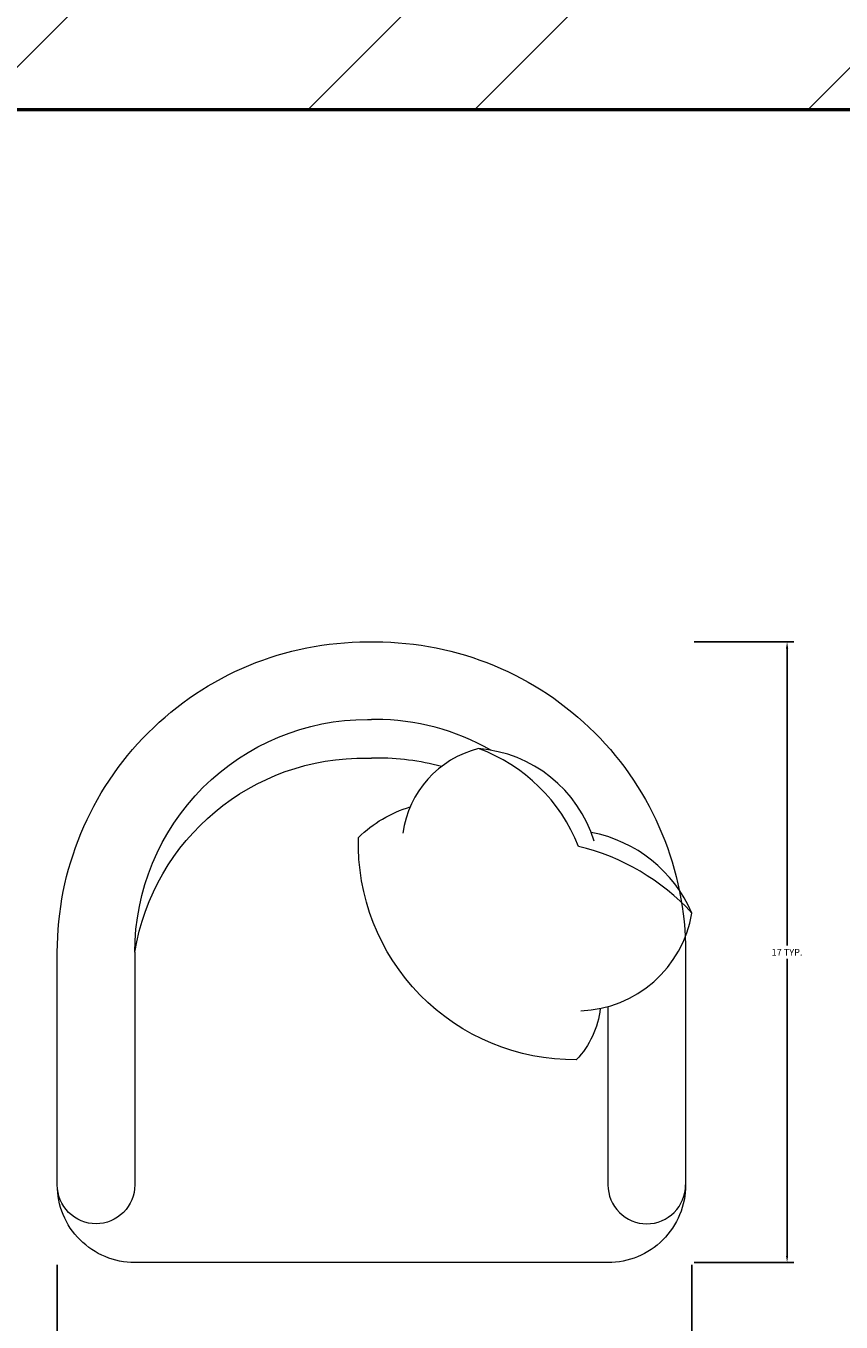
# Model space of a CAD drawing. Units: inches. Extents: x 963 to 2075, y 289 to 2657.
# Tile 78 of 98: x 1467 to 1489, y 2290 to 2325. Entities that reach past the tile are written whole.
import ezdxf

# ---------------------------------------------------------------- set-up
doc = ezdxf.new("R2010")
doc.units = ezdxf.units.IN
for name, color, linetype, lineweight in [('A-ANNO-DIMS', 2, 'Continuous', 18), ('A-FURN', 8, 'Continuous', 18), ('A-WALL', 7, 'Continuous', 50), ('A-WALL-PATT', 8, 'Continuous', 13)]:
    doc.layers.add(name, color=color, linetype=linetype, lineweight=lineweight)
doc.styles.get("Standard").update_dxf_attribs({"font": 'arial.ttf'})
doc.dimstyles.get("Standard").update_dxf_attribs({"dimtxt": 0.18, "dimasz": 0.18, "dimexe": 0.18, "dimexo": 0.0625, "dimgap": 0.09, "dimtad": 0, "dimtih": 1, "dimtoh": 1, "dimdec": 4, "dimzin": 0, "dimdsep": 46, "dimtxsty": 'Standard', "dimcen": 0.09, "dimadec": 0, "dimazin": 0, "dimtfac": 1, "dimtdec": 4, "dimtofl": 0, "dimtmove": 0, "dimatfit": 3, "dimfxl": 1, "dimtolj": 1, "dimtzin": 0, "dimarcsym": 0})

# ---------------------------------------------------------------- blocks, each defined once
blk = doc.blocks.new('ARMCHAIR-B')
at = {"ltscale": 0.03}
blk.add_lwpolyline([(8.888, -0.236), (2.514, -0.236, -0.414214), (0.425, 1.854), (0.425, 8.122, -0.414214), (8.783, 16.481), (8.888, 16.481), (8.992, 16.481, -0.414214), (17.351, 8.122), (17.351, 1.854, -0.414214), (15.261, -0.236), (8.888, -0.236)], format="xyb", dxfattribs=at)
for points in [[(2.514, 8.122, -0.414214), (8.783, 14.391), (8.888, 14.391)], [(12.104, 13.565, 0.130591), (8.992, 14.391), (8.888, 14.391)], [(2.514, 8.122, -0.372719), (8.783, 13.347), (8.888, 13.347)], [(10.774, 13.121, 0.072384), (8.992, 13.347), (8.888, 13.347)], [(14.89, 11.116, 0.306663), (11.774, 13.606, 0.30633), (9.738, 11.332, -0.872847)], [(17.522, 9.177, 0.14773), (14.468, 10.973, 0.213343), (11.774, 13.606, 0.178662)], [(15.054, 6.607, -0.165541), (14.408, 5.227, -0.425989), (8.54, 11.212, -0.121523), (9.933, 12.037, 7.115464)], [(14.528, 6.544, 0.356772), (17.522, 9.177, 0.249542), (14.809, 11.347, -9.61688)], [(2.514, 8.123), (2.514, 1.854, -0.414214), (1.469, 0.809), (1.469, 0.809, -0.414214), (0.425, 1.854)], [(15.261, 6.658), (15.261, 1.854, 0.414214), (16.306, 0.809), (16.306, 0.809, 0.414214), (17.351, 1.854)]]:
    blk.add_lwpolyline(points, format="xyb")
blk = doc.blocks.new('*D24')
at = {"layer": 'A-ANNO-DIMS', "color": 0, "lineweight": -2, "transparency": 16777216}
for p, q in [((1467.425, 2291.701), (1467.425, 2289.019)), ((1484.522, 2291.701), (1484.522, 2289.019)), ((1467.605, 2289.199), (1474.616, 2289.199)), ((1484.342, 2289.199), (1477.331, 2289.199))]:
    blk.add_line(p, q, dxfattribs=at)
at = {"layer": 'A-ANNO-DIMS', "color": 0, "transparency": 16777216}
for points in [[(1467.605, 2289.229), (1467.605, 2289.169), (1467.425, 2289.199)], [(1484.342, 2289.229), (1484.342, 2289.169), (1484.522, 2289.199)]]:
    blk.add_solid(points, dxfattribs=at)
at = {"layer": 'Defpoints', "color": 0, "transparency": 16777216}
for p in [(1467.425, 2291.764), (1484.522, 2291.764), (1484.522, 2289.199)]:
    blk.add_point(p, dxfattribs=at)
at = {"layer": 'A-ANNO-DIMS', "color": 0, "transparency": 16777216, "insert": (1475.973, 2289.199), "char_height": 0.18, "attachment_point": 5}
blk.add_mtext('\\A1;ARMCHAIR B 17 TYP.', dxfattribs=at)
blk = doc.blocks.new('*D25')
at = {"layer": 'A-ANNO-DIMS', "color": 0, "lineweight": -2, "transparency": 16777216}
for p, q in [((1484.584, 2308.481), (1487.266, 2308.481)), ((1487.086, 2308.301), (1487.086, 2300.303)), ((1487.086, 2291.944), (1487.086, 2299.942)), ((1484.584, 2291.764), (1487.266, 2291.764))]:
    blk.add_line(p, q, dxfattribs=at)
at = {"layer": 'A-ANNO-DIMS', "color": 0, "transparency": 16777216}
for points in [[(1487.056, 2308.301), (1487.116, 2308.301), (1487.086, 2308.481)], [(1487.056, 2291.944), (1487.116, 2291.944), (1487.086, 2291.764)]]:
    blk.add_solid(points, dxfattribs=at)
at = {"layer": 'Defpoints', "color": 0, "transparency": 16777216}
for p in [(1484.522, 2308.481), (1487.086, 2308.481), (1484.522, 2291.764)]:
    blk.add_point(p, dxfattribs=at)
at = {"layer": 'A-ANNO-DIMS', "color": 0, "transparency": 16777216, "insert": (1487.086, 2300.122), "char_height": 0.18, "attachment_point": 5}
blk.add_mtext('\\A1;17 TYP.', dxfattribs=at)

msp = doc.modelspace()

# ---------------------------------------------------------------- hatches: boundary and pattern name
at = {"layer": 'A-WALL-PATT'}
h = msp.add_hatch(dxfattribs=at)
h.set_pattern_fill('ANSI32', color=256)
h.paths.add_polyline_path([(1296.922, 2558.318), (1203.922, 2558.318), (1203.922, 2493.818), (1191.533, 2493.818), (1191.533, 2489.318), (1211.063, 2489.318), (1211.063, 2492.02), (1211.063, 2493.818), (1208.422, 2493.818), (1208.422, 2553.818), (1292.422, 2553.818), (1292.422, 2538.863), (1296.922, 2538.863)])
h.paths.add_polyline_path([(1442.422, 2558.318), (1349.422, 2558.318), (1349.422, 2538.943), (1353.922, 2538.943), (1353.922, 2553.818), (1437.922, 2553.818), (1437.922, 2493.818), (1434.542, 2493.818), (1434.542, 2489.318), (1448.311, 2489.318), (1448.311, 2491.568), (1448.311, 2493.818), (1442.422, 2493.818)])
h.paths.add_polyline_path([(1415.554, 2491.568), (1415.554, 2493.818), (1340.941, 2493.818), (1340.941, 2489.318), (1371.922, 2489.318), (1371.922, 2378.318), (1367.596, 2378.318), (1367.596, 2373.818), (1371.922, 2373.818), (1371.922, 2355.185), (1376.422, 2355.185), (1376.422, 2489.318), (1415.554, 2489.318)])
h.paths.add_polyline_path([(1304.941, 2491.568), (1304.941, 2493.818), (1296.922, 2493.818), (1296.922, 2514.863), (1292.422, 2514.863), (1292.422, 2493.818), (1232.808, 2493.818), (1232.808, 2489.318), (1256.422, 2489.318), (1256.422, 2327.318), (1253.714, 2327.318), (1253.714, 2322.818), (1328.422, 2322.818), (1328.422, 2331.147), (1323.922, 2331.147), (1323.922, 2327.318), (1260.922, 2327.318), (1260.922, 2373.818), (1323.922, 2373.818), (1323.922, 2357.812), (1328.422, 2357.812), (1328.422, 2373.818), (1346.007, 2373.818), (1346.007, 2376.068), (1346.007, 2378.318), (1260.922, 2378.318), (1260.922, 2489.318), (1304.941, 2489.318)])
h.paths.add_polyline_path([(1226.654, 2327.318), (1124.422, 2327.318), (1124.422, 2347.447), (1119.922, 2347.447), (1119.922, 2322.818), (1163.422, 2322.818), (1163.422, 2305.435), (1165.672, 2305.435), (1167.922, 2305.435), (1167.922, 2322.818), (1226.654, 2322.818), (1226.654, 2325.068)])
h.paths.add_polyline_path([(1095.922, 2489.318), (1124.422, 2489.318), (1131.533, 2489.318), (1131.533, 2491.568), (1131.533, 2493.818), (1119.922, 2493.818), (1091.422, 2493.818), (1091.422, 2417.318), (1095.922, 2417.318), (1119.922, 2417.318), (1119.922, 2407.447), (1124.422, 2407.447), (1124.422, 2421.818), (1095.922, 2421.818)])
h.paths.add_polyline_path([(1512.922, 2558.318), (1508.422, 2558.318), (1508.422, 2493.818), (1503.401, 2493.818), (1503.401, 2489.318), (1508.422, 2489.318), (1508.422, 2327.318), (1376.422, 2327.318), (1376.422, 2330.273), (1371.922, 2330.273), (1371.922, 2298.744), (1376.422, 2298.744), (1376.422, 2322.818), (1508.422, 2322.818), (1508.422, 2165.318), (1504.255, 2165.318), (1504.255, 2160.818), (1508.422, 2160.818), (1508.422, 2108.318), (1512.922, 2108.318), (1512.922, 2160.818), (1516.182, 2160.818), (1516.182, 2163.068), (1516.182, 2165.318), (1512.922, 2165.318), (1512.922, 2322.818), (1644.922, 2322.818), (1644.922, 2298.744), (1649.422, 2298.744), (1649.422, 2322.818), (1649.422, 2330.944), (1647.172, 2330.944), (1644.922, 2330.944), (1644.922, 2327.318), (1512.922, 2327.318), (1512.922, 2489.318), (1516.759, 2489.318), (1516.759, 2491.568), (1516.759, 2493.818), (1512.922, 2493.818)])
h.paths.add_polyline_path([(1671.922, 2558.318), (1578.922, 2558.318), (1578.922, 2493.818), (1573.526, 2493.818), (1573.526, 2489.318), (1586.537, 2489.318), (1586.537, 2491.568), (1586.537, 2493.818), (1583.422, 2493.818), (1583.422, 2553.818), (1667.422, 2553.818), (1667.422, 2541.109), (1671.922, 2541.109)])
h.paths.add_polyline_path([(1681.257, 2493.818), (1671.922, 2493.818), (1671.922, 2517.109), (1667.422, 2517.109), (1667.422, 2493.818), (1610.218, 2493.818), (1610.218, 2489.318), (1644.922, 2489.318), (1644.922, 2357.865), (1649.422, 2357.865), (1649.422, 2373.818), (1652.203, 2373.818), (1652.203, 2375.827), (1652.203, 2378.318), (1649.422, 2378.318), (1649.422, 2489.318), (1681.257, 2489.318), (1681.257, 2491.568)])
h.paths.add_polyline_path([(1821.922, 2558.318), (1728.922, 2558.318), (1728.922, 2541), (1733.422, 2541), (1733.422, 2553.818), (1817.422, 2553.818), (1817.422, 2493.818), (1813.507, 2493.818), (1813.507, 2489.318), (1830.078, 2489.318), (1830.078, 2491.568), (1830.078, 2493.818), (1821.922, 2493.818)])
h.paths.add_polyline_path([(1794.244, 2493.818), (1717.257, 2493.818), (1717.257, 2489.318), (1760.422, 2489.318), (1760.422, 2378.318), (1674.401, 2378.318), (1674.401, 2373.818), (1692.922, 2373.818), (1692.922, 2356.954), (1697.422, 2356.954), (1697.422, 2373.818), (1760.422, 2373.818), (1760.422, 2327.318), (1697.422, 2327.318), (1697.422, 2333.341), (1692.922, 2333.341), (1692.922, 2322.818), (1768.037, 2322.818), (1768.037, 2325.068), (1768.037, 2327.318), (1764.922, 2327.318), (1764.922, 2489.318), (1794.244, 2489.318)])
h.paths.add_polyline_path([(1733.422, 2517), (1728.922, 2517), (1728.922, 2493.818), (1733.422, 2493.818)], flags=17)
h.paths.add_polyline_path([(1929.922, 2493.818), (1890.078, 2493.818), (1890.078, 2489.318), (1896.922, 2489.318), (1925.422, 2489.318), (1925.422, 2421.818), (1896.922, 2421.818), (1896.922, 2408.318), (1901.422, 2408.318), (1901.422, 2417.318), (1925.422, 2417.318), (1929.922, 2417.318)])
h.paths.add_polyline_path([(1901.422, 2348.318), (1896.922, 2348.318), (1896.922, 2327.318), (1800.423, 2327.318), (1800.423, 2322.818), (1853.422, 2322.818), (1853.422, 2309.453), (1857.922, 2309.453), (1857.922, 2322.818), (1901.422, 2322.818)])
h.paths.add_polyline_path([(1857.922, 2249.453), (1853.422, 2249.453), (1853.422, 2214.818), (1686.309, 2214.818), (1686.309, 2210.318), (1853.422, 2210.318), (1853.422, 2202.134), (1857.922, 2202.134), (1857.922, 2210.318)])
h.paths.add_polyline_path([(1857.922, 2142.134), (1853.422, 2142.134), (1853.422, 2115.422), (1841.422, 2115.422), (1841.422, 2088.531), (1841.422, 2046.949), (1845.922, 2046.949), (1845.922, 2110.922), (1905.922, 2110.922), (1905.922, 2092.517), (1910.422, 2092.517), (1910.422, 2115.422), (1857.922, 2115.422)])
h.paths.add_polyline_path([(1532.436, 1482.342), (1573.456, 1482.342), (1573.456, 1501), (1532.436, 1501)], flags=9)
h.paths.add_polyline_path([(1438.658, 1486.302), (1479.678, 1486.302), (1479.678, 1504.96), (1438.658, 1504.96)], flags=9)
h.paths.add_polyline_path([(1411.215, 1365.308), (1659.139, 1365.308), (1659.139, 1402.401), (1411.215, 1402.401)], flags=9)
h.paths.add_polyline_path([(1185.671, 2296.298), (1248.16, 2296.298), (1248.16, 2314.955), (1185.671, 2314.955)], flags=9)
h.paths.add_polyline_path([(1177.31, 2187.35), (1216.15, 2187.35), (1216.15, 2206.007), (1177.31, 2206.007)], flags=9)
h.paths.add_polyline_path([(1295.101, 1602.083), (1328.26, 1602.083), (1328.26, 1620.741), (1295.101, 1620.741)], flags=9)
h.paths.add_polyline_path([(1525.126, 2005.99), (1558.39, 2005.99), (1558.39, 2024.648), (1525.126, 2024.648)], flags=9)
h.paths.add_polyline_path([(1459.606, 1977.125), (1472.195, 1977.125), (1472.195, 1987.429), (1459.606, 1987.429)], flags=9)
h.paths.add_polyline_path([(1467.815, 2053.676), (1480.018, 2053.676), (1480.018, 2063.979), (1467.815, 2063.979)], flags=9)
h.paths.add_polyline_path([(1555.184, 2119.02), (1584.563, 2119.02), (1584.563, 2137.678), (1555.184, 2137.678)], flags=25)
h.paths.add_polyline_path([(1405.389, 2115.291), (1444.478, 2115.291), (1444.478, 2133.948), (1405.389, 2133.948)], flags=25)
h.paths.add_polyline_path([(1698.482, 2004.259), (1727.695, 2004.259), (1727.695, 2022.916), (1698.482, 2022.916)], flags=9)
h.paths.add_polyline_path([(1612.158, 1972.855), (1629.016, 1972.855), (1629.016, 1983.159), (1612.158, 1983.159)], flags=9)
h.paths.add_polyline_path([(1608.289, 2060.036), (1625.147, 2060.036), (1625.147, 2070.34), (1608.289, 2070.34)], flags=9)
h.paths.add_polyline_path([(1527.954, 1684.402), (1566.795, 1684.402), (1566.795, 1703.06), (1527.954, 1703.06)], flags=9)
h.paths.add_polyline_path([(1422.792, 1683.59), (1461.633, 1683.59), (1461.633, 1702.247), (1422.792, 1702.247)], flags=9)
h.paths.add_polyline_path([(1531.262, 1732.459), (1574.015, 1732.459), (1574.015, 1751.116), (1531.262, 1751.116)], flags=9)
h.paths.add_polyline_path([(1402.872, 1732.845), (1439.799, 1732.845), (1439.799, 1751.502), (1402.872, 1751.502)], flags=9)
h.paths.add_polyline_path([(1243.122, 1923.132), (1281.962, 1923.132), (1281.962, 1941.79), (1243.122, 1941.79)], flags=9)
h.paths.add_polyline_path([(1181.752, 1792.268), (1244.241, 1792.268), (1244.241, 1810.926), (1181.752, 1810.926)], flags=9)
h.paths.add_polyline_path([(1265.822, 1670.3), (1316.071, 1670.3), (1316.071, 1688.957), (1265.822, 1688.957)], flags=9)
h.paths.add_polyline_path([(1140.263, 1676.054), (1179.104, 1676.054), (1179.104, 1694.711), (1140.263, 1694.711)], flags=9)
h.paths.add_polyline_path([(1107.49, 1490.889), (1143.374, 1490.889), (1143.374, 1509.546), (1107.49, 1509.546)], flags=9)
h.paths.add_polyline_path([(1217.584, 1483.899), (1246.741, 1483.899), (1246.741, 1502.556), (1217.584, 1502.556)], flags=9)
h.paths.add_polyline_path([(1389.21, 1486.919), (1418.367, 1486.919), (1418.367, 1505.576), (1389.21, 1505.576)], flags=9)
h.paths.add_polyline_path([(1672.208, 1602.083), (1705.366, 1602.083), (1705.366, 1620.741), (1672.208, 1620.741)], flags=9)
h.paths.add_polyline_path([(1752.082, 1522.638), (1781.24, 1522.638), (1781.24, 1541.295), (1752.082, 1541.295)], flags=9)
h.paths.add_polyline_path([(1848.275, 1491.26), (1884.158, 1491.26), (1884.158, 1509.918), (1848.275, 1509.918)], flags=9)
h.paths.add_polyline_path([(1822.47, 1685.62), (1861.31, 1685.62), (1861.31, 1704.278), (1822.47, 1704.278)], flags=9)
h.paths.add_polyline_path([(1713.195, 1672.232), (1763.444, 1672.232), (1763.444, 1690.889), (1713.195, 1690.889)], flags=9)
h.paths.add_polyline_path([(1736.619, 1790.578), (1799.109, 1790.578), (1799.109, 1809.235), (1736.619, 1809.235)], flags=9)
h.paths.add_polyline_path([(1691.491, 1916.355), (1730.332, 1916.355), (1730.332, 1935.013), (1691.491, 1935.013)], flags=9)
h.paths.add_polyline_path([(1764.872, 1973.922), (1794.306, 1973.922), (1794.306, 1992.58), (1764.872, 1992.58)], flags=9)
h.paths.add_polyline_path([(1767.854, 2034.017), (1797.288, 2034.017), (1797.288, 2052.674), (1767.854, 2052.674)], flags=9)
h.paths.add_polyline_path([(1851.593, 2060.331), (1880.751, 2060.331), (1880.751, 2078.989), (1851.593, 2078.989)], flags=25)
h.paths.add_polyline_path([(1688.491, 2086.874), (1727.332, 2086.874), (1727.332, 2105.531), (1688.491, 2105.531)], flags=9)
h.paths.add_polyline_path([(1537.743, 2293.581), (1580.495, 2293.581), (1580.495, 2312.239), (1537.743, 2312.239)], flags=25)
h.paths.add_polyline_path([(1425.587, 2296.109), (1468.34, 2296.109), (1468.34, 2314.766), (1425.587, 2314.766)], flags=25)
h.paths.add_polyline_path([(1278.518, 2004.184), (1307.72, 2004.184), (1307.72, 2022.841), (1278.518, 2022.841)], flags=9)
h.paths.add_polyline_path([(1193.282, 1973.635), (1222.715, 1973.635), (1222.715, 1992.292), (1193.282, 1992.292)], flags=9)
h.paths.add_polyline_path([(1192.411, 2040.577), (1221.845, 2040.577), (1221.845, 2059.234), (1192.411, 2059.234)], flags=9)
h.paths.add_polyline_path([(1130.603, 1951.393), (1159.76, 1951.393), (1159.76, 1970.05), (1130.603, 1970.05)], flags=9)
h.paths.add_polyline_path([(1132.827, 2052.494), (1161.984, 2052.494), (1161.984, 2071.151), (1132.827, 2071.151)], flags=9)
h.paths.add_polyline_path([(1265.128, 2334.619), (1315.377, 2334.619), (1315.377, 2353.277), (1265.128, 2353.277)], flags=25)
h.paths.add_polyline_path([(1136.741, 2330.785), (1175.582, 2330.785), (1175.582, 2349.443), (1136.741, 2349.443)], flags=9)
h.paths.add_polyline_path([(1287.422, 2417.204), (1320.58, 2417.204), (1320.58, 2435.861), (1287.422, 2435.861)], flags=25)
h.paths.add_polyline_path([(1430.988, 2329.159), (1469.828, 2329.159), (1469.828, 2347.816), (1430.988, 2347.816)], flags=25)
h.paths.add_polyline_path([(1525.424, 2329.213), (1564.264, 2329.213), (1564.264, 2347.87), (1525.424, 2347.87)], flags=25)
h.paths.add_polyline_path([(1684.525, 2382.799), (1717.683, 2382.799), (1717.683, 2401.457), (1684.525, 2401.457)], flags=25)
h.paths.add_polyline_path([(1704.805, 2340.293), (1755.054, 2340.293), (1755.054, 2358.95), (1704.805, 2358.95)], flags=25)
h.paths.add_polyline_path([(1694.113, 2287.757), (1756.602, 2287.757), (1756.602, 2306.414), (1694.113, 2306.414)], flags=9)
h.paths.add_polyline_path([(1815.778, 2329.861), (1854.618, 2329.861), (1854.618, 2348.518), (1815.778, 2348.518)], flags=9)
h.paths.add_polyline_path([(1842.873, 2514.256), (1878.756, 2514.256), (1878.756, 2532.914), (1842.873, 2532.914)], flags=9)
h.paths.add_polyline_path([(1769.513, 2531.447), (1798.671, 2531.447), (1798.671, 2550.104), (1769.513, 2550.104)], flags=25)
h.paths.add_polyline_path([(1594.772, 2518.468), (1623.93, 2518.468), (1623.93, 2537.125), (1594.772, 2537.125)], flags=25)
h.paths.add_polyline_path([(1520.723, 2516.185), (1556.606, 2516.185), (1556.606, 2534.842), (1520.723, 2534.842)], flags=25)
h.paths.add_polyline_path([(1464.456, 2516.694), (1500.34, 2516.694), (1500.34, 2535.351), (1464.456, 2535.351)], flags=25)
h.paths.add_polyline_path([(1365.696, 2528.97), (1394.854, 2528.97), (1394.854, 2547.627), (1365.696, 2547.627)], flags=25)
h.paths.add_polyline_path([(1222.838, 2516.231), (1251.995, 2516.231), (1251.995, 2534.889), (1222.838, 2534.889)], flags=25)
h.paths.add_polyline_path([(1104.545, 2509.6), (1140.429, 2509.6), (1140.429, 2528.257), (1104.545, 2528.257)], flags=9)
h = msp.add_hatch(dxfattribs=at)
h.set_pattern_fill('ANSI32', color=256)
h.paths.add_polyline_path([(1335.968, 2212.568), (1335.968, 2214.818), (1167.922, 2214.818), (1167.922, 2245.435), (1163.422, 2245.435), (1163.422, 2210.318), (1163.422, 2194.812), (1167.922, 2194.812), (1167.922, 2210.318), (1335.968, 2210.318)])
h.paths.add_polyline_path([(1532.436, 1482.342), (1573.456, 1482.342), (1573.456, 1501), (1532.436, 1501)], flags=9)
h.paths.add_polyline_path([(1438.658, 1486.302), (1479.678, 1486.302), (1479.678, 1504.96), (1438.658, 1504.96)], flags=9)
h.paths.add_polyline_path([(1411.215, 1365.308), (1659.139, 1365.308), (1659.139, 1402.401), (1411.215, 1402.401)], flags=9)
h.paths.add_polyline_path([(1185.671, 2296.298), (1248.16, 2296.298), (1248.16, 2314.955), (1185.671, 2314.955)], flags=9)
h.paths.add_polyline_path([(1177.31, 2187.35), (1216.15, 2187.35), (1216.15, 2206.007), (1177.31, 2206.007)], flags=9)
h.paths.add_polyline_path([(1295.101, 1602.083), (1328.26, 1602.083), (1328.26, 1620.741), (1295.101, 1620.741)], flags=9)
h.paths.add_polyline_path([(1525.126, 2005.99), (1558.39, 2005.99), (1558.39, 2024.648), (1525.126, 2024.648)], flags=9)
h.paths.add_polyline_path([(1459.606, 1977.125), (1472.195, 1977.125), (1472.195, 1987.429), (1459.606, 1987.429)], flags=9)
h.paths.add_polyline_path([(1467.815, 2053.676), (1480.018, 2053.676), (1480.018, 2063.979), (1467.815, 2063.979)], flags=9)
h.paths.add_polyline_path([(1555.184, 2119.02), (1584.563, 2119.02), (1584.563, 2137.678), (1555.184, 2137.678)], flags=9)
h.paths.add_polyline_path([(1405.389, 2115.291), (1444.478, 2115.291), (1444.478, 2133.948), (1405.389, 2133.948)], flags=9)
h.paths.add_polyline_path([(1698.482, 2004.259), (1727.695, 2004.259), (1727.695, 2022.916), (1698.482, 2022.916)], flags=9)
h.paths.add_polyline_path([(1612.158, 1972.855), (1629.016, 1972.855), (1629.016, 1983.159), (1612.158, 1983.159)], flags=9)
h.paths.add_polyline_path([(1608.289, 2060.036), (1625.147, 2060.036), (1625.147, 2070.34), (1608.289, 2070.34)], flags=9)
h.paths.add_polyline_path([(1527.954, 1684.402), (1566.795, 1684.402), (1566.795, 1703.06), (1527.954, 1703.06)], flags=9)
h.paths.add_polyline_path([(1422.792, 1683.59), (1461.633, 1683.59), (1461.633, 1702.247), (1422.792, 1702.247)], flags=9)
h.paths.add_polyline_path([(1531.262, 1732.459), (1574.015, 1732.459), (1574.015, 1751.116), (1531.262, 1751.116)], flags=9)
h.paths.add_polyline_path([(1402.872, 1732.845), (1439.799, 1732.845), (1439.799, 1751.502), (1402.872, 1751.502)], flags=9)
h.paths.add_polyline_path([(1243.122, 1923.132), (1281.962, 1923.132), (1281.962, 1941.79), (1243.122, 1941.79)], flags=9)
h.paths.add_polyline_path([(1181.752, 1792.268), (1244.241, 1792.268), (1244.241, 1810.926), (1181.752, 1810.926)], flags=9)
h.paths.add_polyline_path([(1265.822, 1670.3), (1316.071, 1670.3), (1316.071, 1688.957), (1265.822, 1688.957)], flags=9)
h.paths.add_polyline_path([(1140.263, 1676.054), (1179.104, 1676.054), (1179.104, 1694.711), (1140.263, 1694.711)], flags=9)
h.paths.add_polyline_path([(1107.49, 1490.889), (1143.374, 1490.889), (1143.374, 1509.546), (1107.49, 1509.546)], flags=9)
h.paths.add_polyline_path([(1217.584, 1483.899), (1246.741, 1483.899), (1246.741, 1502.556), (1217.584, 1502.556)], flags=9)
h.paths.add_polyline_path([(1389.21, 1486.919), (1418.367, 1486.919), (1418.367, 1505.576), (1389.21, 1505.576)], flags=9)
h.paths.add_polyline_path([(1672.208, 1602.083), (1705.366, 1602.083), (1705.366, 1620.741), (1672.208, 1620.741)], flags=9)
h.paths.add_polyline_path([(1752.082, 1522.638), (1781.24, 1522.638), (1781.24, 1541.295), (1752.082, 1541.295)], flags=9)
h.paths.add_polyline_path([(1848.275, 1491.26), (1884.158, 1491.26), (1884.158, 1509.918), (1848.275, 1509.918)], flags=9)
h.paths.add_polyline_path([(1822.47, 1685.62), (1861.31, 1685.62), (1861.31, 1704.278), (1822.47, 1704.278)], flags=9)
h.paths.add_polyline_path([(1713.195, 1672.232), (1763.444, 1672.232), (1763.444, 1690.889), (1713.195, 1690.889)], flags=9)
h.paths.add_polyline_path([(1736.619, 1790.578), (1799.109, 1790.578), (1799.109, 1809.235), (1736.619, 1809.235)], flags=9)
h.paths.add_polyline_path([(1691.491, 1916.355), (1730.332, 1916.355), (1730.332, 1935.013), (1691.491, 1935.013)], flags=9)
h.paths.add_polyline_path([(1764.872, 1973.922), (1794.306, 1973.922), (1794.306, 1992.58), (1764.872, 1992.58)], flags=9)
h.paths.add_polyline_path([(1767.854, 2034.017), (1797.288, 2034.017), (1797.288, 2052.674), (1767.854, 2052.674)], flags=9)
h.paths.add_polyline_path([(1851.593, 2060.331), (1880.751, 2060.331), (1880.751, 2078.989), (1851.593, 2078.989)], flags=9)
h.paths.add_polyline_path([(1688.491, 2086.874), (1727.332, 2086.874), (1727.332, 2105.531), (1688.491, 2105.531)], flags=9)
h.paths.add_polyline_path([(1537.743, 2293.581), (1580.495, 2293.581), (1580.495, 2312.239), (1537.743, 2312.239)], flags=9)
h.paths.add_polyline_path([(1425.587, 2296.109), (1468.34, 2296.109), (1468.34, 2314.766), (1425.587, 2314.766)], flags=9)
h.paths.add_polyline_path([(1278.518, 2004.184), (1307.72, 2004.184), (1307.72, 2022.841), (1278.518, 2022.841)], flags=9)
h.paths.add_polyline_path([(1193.282, 1973.635), (1222.715, 1973.635), (1222.715, 1992.292), (1193.282, 1992.292)], flags=9)
h.paths.add_polyline_path([(1192.411, 2040.577), (1221.845, 2040.577), (1221.845, 2059.234), (1192.411, 2059.234)], flags=9)
h.paths.add_polyline_path([(1130.603, 1951.393), (1159.76, 1951.393), (1159.76, 1970.05), (1130.603, 1970.05)], flags=9)
h.paths.add_polyline_path([(1132.827, 2052.494), (1161.984, 2052.494), (1161.984, 2071.151), (1132.827, 2071.151)], flags=9)
h.paths.add_polyline_path([(1265.128, 2334.619), (1315.377, 2334.619), (1315.377, 2353.277), (1265.128, 2353.277)], flags=9)
h.paths.add_polyline_path([(1136.741, 2330.785), (1175.582, 2330.785), (1175.582, 2349.443), (1136.741, 2349.443)], flags=9)
h.paths.add_polyline_path([(1287.422, 2417.204), (1320.58, 2417.204), (1320.58, 2435.861), (1287.422, 2435.861)], flags=9)
h.paths.add_polyline_path([(1430.988, 2329.159), (1469.828, 2329.159), (1469.828, 2347.816), (1430.988, 2347.816)], flags=9)
h.paths.add_polyline_path([(1525.424, 2329.213), (1564.264, 2329.213), (1564.264, 2347.87), (1525.424, 2347.87)], flags=9)
h.paths.add_polyline_path([(1684.525, 2382.799), (1717.683, 2382.799), (1717.683, 2401.457), (1684.525, 2401.457)], flags=9)
h.paths.add_polyline_path([(1704.805, 2340.293), (1755.054, 2340.293), (1755.054, 2358.95), (1704.805, 2358.95)], flags=9)
h.paths.add_polyline_path([(1694.113, 2287.757), (1756.602, 2287.757), (1756.602, 2306.414), (1694.113, 2306.414)], flags=9)
h.paths.add_polyline_path([(1815.778, 2329.861), (1854.618, 2329.861), (1854.618, 2348.518), (1815.778, 2348.518)], flags=9)
h.paths.add_polyline_path([(1842.873, 2514.256), (1878.756, 2514.256), (1878.756, 2532.914), (1842.873, 2532.914)], flags=9)
h.paths.add_polyline_path([(1769.513, 2531.447), (1798.671, 2531.447), (1798.671, 2550.104), (1769.513, 2550.104)], flags=9)
h.paths.add_polyline_path([(1594.772, 2518.468), (1623.93, 2518.468), (1623.93, 2537.125), (1594.772, 2537.125)], flags=9)
h.paths.add_polyline_path([(1520.723, 2516.185), (1556.606, 2516.185), (1556.606, 2534.842), (1520.723, 2534.842)], flags=9)
h.paths.add_polyline_path([(1464.456, 2516.694), (1500.34, 2516.694), (1500.34, 2535.351), (1464.456, 2535.351)], flags=9)
h.paths.add_polyline_path([(1365.696, 2528.97), (1394.854, 2528.97), (1394.854, 2547.627), (1365.696, 2547.627)], flags=9)
h.paths.add_polyline_path([(1222.838, 2516.231), (1251.995, 2516.231), (1251.995, 2534.889), (1222.838, 2534.889)], flags=9)
h.paths.add_polyline_path([(1104.545, 2509.6), (1140.429, 2509.6), (1140.429, 2528.257), (1104.545, 2528.257)], flags=9)

# ---------------------------------------------------------------- linework, layer by layer
at = {"layer": 'A-WALL'}
msp.add_line((1376.422, 2322.818), (1508.422, 2322.818), dxfattribs=at)

# ---------------------------------------------------------------- block references
at = {"layer": 'A-FURN'}
msp.add_blockref('ARMCHAIR-B', (1467, 2292), dxfattribs=at)

# ---------------------------------------------------------------- dimensions: what is measured, and where the dimension line sits
at = {"layer": 'A-ANNO-DIMS'}
dim = msp.add_linear_dim(base=(1487.086, 2308.481), p1=(1484.522, 2291.764), p2=(1484.522, 2308.481), angle=90, text='<> TYP.', dimstyle='Standard', override={"dimdec": 0, "dimlfac": 1, "dimrnd": 0, "dimzin": 0, "dimdsep": 46, "dimlunit": 2}, dxfattribs=at)
dim.commit()
dim.dimension.update_dxf_attribs({"geometry": '*D25', "text_midpoint": (1487.086, 2300.122)})
dim = msp.add_linear_dim(base=(1484.522, 2289.199), p1=(1467.425, 2291.764), p2=(1484.522, 2291.764), text='ARMCHAIR B <> TYP.', dimstyle='Standard', override={"dimdec": 0, "dimlfac": 1, "dimrnd": 0, "dimzin": 0, "dimdsep": 46, "dimlunit": 2}, dxfattribs=at)
dim.commit()
dim.dimension.update_dxf_attribs({"geometry": '*D24', "text_midpoint": (1475.973, 2289.199)})

doc.saveas('drawing.dxf')
